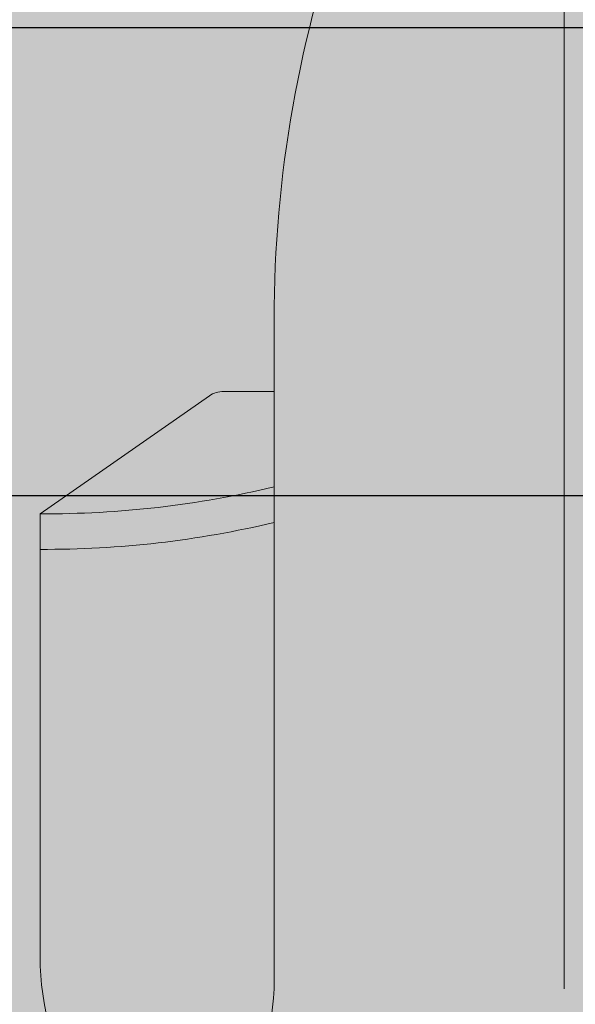
# Model space of a CAD drawing. Units: inches. Extents: x 389 to 971, y 148 to 870.
# Tile 2 of 14: x 500 to 515, y 364 to 389. Entities that reach past the tile are written whole.
import ezdxf

# ---------------------------------------------------------------- set-up
doc = ezdxf.new("R2010")
doc.units = ezdxf.units.IN
doc.header["$MEASUREMENT"] = 0
for name, color, linetype, lineweight in [('A-ANNO-DIMS', 2, 'Continuous', 18), ('C-VEHI', 8, 'Continuous', 13), ('L-GRND-BASE-PATT', 8, 'Continuous', 13)]:
    doc.layers.add(name, color=color, linetype=linetype, lineweight=lineweight)
doc.layers.add('C-VEHI-PATT', color=18, linetype='Continuous', lineweight=13, true_color=0x000000)
doc.layers.add('L-GRND-PATT', color=39, linetype='Continuous', lineweight=13, true_color=0x603913)
doc.styles.get("Standard").update_dxf_attribs({"font": 'arial.ttf'})
doc.dimstyles.get("Standard").update_dxf_attribs({"dimtxt": 8, "dimasz": 8, "dimexe": 0.18, "dimexo": 0.0625, "dimgap": 0.09, "dimtad": 0, "dimtih": 1, "dimtoh": 1, "dimdec": 0, "dimzin": 0, "dimdsep": 46, "dimlunit": 3, "dimtxsty": 'Standard', "dimcen": 0.09, "dimadec": 0, "dimazin": 0, "dimtfac": 1, "dimtdec": 0, "dimtofl": 0, "dimtmove": 0, "dimatfit": 3, "dimfxl": 1, "dimtolj": 1, "dimtzin": 0, "dimarcsym": 0})

# ---------------------------------------------------------------- blocks, each defined once
blk = doc.blocks.new('*U7')
for p, q in [((-4.43e-14, -2.558e-13), (51.68362801571248, -2.558e-13)), ((29.77279020470884, -9.50583338362054), (51.68362801571248, -9.50583338362054)), ((32.12291633764599, -9.50583338362054), (32.12291633764599, -11.15369945057762)), ((32.26591480791686, -11.62530558863292), (36.12873726252356, -17.16961494239257)), ((36.12873726252356, -17.16961494239257), (50.93891189819171, -17.16961494239257))]:
    blk.add_line(p, q)
for centre, major_axis, ratio, start_param, end_param in [((29.77279020470884, -46.66302566589627), (5.12e-14, 56.16885904951626), 0.842303869543976, 7e-16, 0.5903187773915901), ((29.77279020470884, 46.66302566589578), (4.004e-13, 56.16885904951626), 0.8423038695439734, 2.55127387619821, 3.141592653589801), ((13.03653510440275, -17.00972444508983), (1.2568e-12, -27.41599049210552), 0.8423038695439318, 1.564964277657711, 1.848039256919935), ((14.20086229321332, -17.00972444508983), (1.2568e-12, -27.41599049210552), 0.8423038695439318, 1.564964277657711, 1.848039256919935), ((32.74615637525823, -11.1536994505777), (1.3e-13, -0.7399230374541176), 0.8423038695439093, 4.712388980384541, 5.403471737230034)]:
    blk.add_ellipse(centre, major_axis=major_axis, ratio=ratio, start_param=start_param, end_param=end_param)
at = {"extrusion": (0, 0, -1)}
blk.add_ellipse((50.7902773840875, -13.33772416300655), major_axis=(6.340077547122382, 0.3566085810370246), ratio=0.6038335755719145, start_param=-1.39555193967809, end_param=1.581314658479915, dxfattribs=at)
blk = doc.blocks.new('*D53')
at = {"layer": 'A-ANNO-DIMS', "color": 0, "lineweight": -2, "transparency": 16777216}
for p, q in [((397.8910240000004, 396.9189020000002), (397.8910240000004, 404.9189020000001)), ((690.1535240000002, 388.9189020000003), (397.7110240000004, 388.9189020000002)), ((690.1535240000002, 376.9189020000001), (397.7110240000005, 376.9189020000001)), ((397.8910240000005, 368.9189020000001), (397.8910240000005, 360.918902))]:
    blk.add_line(p, q, dxfattribs=at)
at = {"layer": 'A-ANNO-DIMS', "color": 0, "transparency": 16777216}
for points in [[(396.5576906666671, 396.9189020000002), (399.2243573333337, 396.9189020000002), (397.8910240000004, 388.9189020000002)], [(396.5576906666671, 368.9189020000001), (399.2243573333338, 368.9189020000001), (397.8910240000005, 376.9189020000001)]]:
    blk.add_solid(points, dxfattribs=at)
at = {"layer": 'Defpoints', "color": 0, "transparency": 16777216}
for p in [(397.8910240000004, 388.9189020000002), (690.2160240000001, 388.9189020000003), (690.2160240000001, 376.9189020000001)]:
    blk.add_point(p, dxfattribs=at)
at = {"layer": 'A-ANNO-DIMS', "color": 0, "transparency": 16777216, "insert": (397.8910240000004, 382.9189019999999), "char_height": 8, "attachment_point": 5}
blk.add_mtext('\\A1;12', dxfattribs=at)

msp = doc.modelspace()

# ---------------------------------------------------------------- hatches: boundary and pattern name
at = {"layer": 'C-VEHI-PATT'}
h = msp.add_hatch(color=256, dxfattribs=at)
h.dxf.hatch_style = 1
edge = h.paths.add_edge_path()
edge.add_ellipse((550.9021553826709, 381.4331108862803), major_axis=(-43.99405423656321, 1.9369e-12), ratio=0.8423038695439613, start_angle=-29.43856959797762, end_angle=1.8189894035458565e-12, ccw=False)
edge.add_line((514.3535105156315, 402.059641051582), (514.3535105156315, 404.7525403567118))
edge.add_ellipse((514.3535105156316, 404.2643898676136), major_axis=(0.5795420236673633, 2e-16), ratio=0.8423038695437671, start_angle=90.00000000001334, end_angle=127.9331304598466)
edge.add_line((514.0354569934393, 404.6724605914631), (509.5535496243029, 402.1940957519602))
edge.add_ellipse((473.3138688667988, 564.9222417143382), major_axis=(196.5636751472093, 8.4793e-12), ratio=0.8423038695439335, start_angle=-80.7434339928015, end_angle=-77.44506735586577, ccw=False)
edge.add_ellipse((535.9119176052684, 201.7546502845751), major_axis=(239.1273775699096, 1.008988e-10), ratio=0.842303869543627, start_angle=100.2095389971183, end_angle=102.4446272934191)
edge.add_ellipse((979.5722266908713, 375.4013592680145), major_axis=(-488.2195497741742, 7.7268e-12), ratio=0.842303869543895, start_angle=-2.863714607837472, end_angle=2.198540565955285)
edge.add_ellipse((510.1338164488812, 299.4839331720496), major_axis=(70.3178640738586, 3.814e-12), ratio=0.8423038695439212, start_angle=94.08241069114638, end_angle=107.71995322274631, ccw=False)
edge.add_line((505.914122382133, 358.6062023341113), (522.79289864913, 358.606202334111))
edge.add_ellipse((518.5732045823792, 299.4839331720493), major_axis=(-70.31786407385354, 1.4408e-12), ratio=0.8423038695439844, start_angle=252.2800467772501, end_angle=265.91758930884987, ccw=False)
edge.add_ellipse((49.13479434038987, 375.4013592680261), major_axis=(-488.2195497741754, 2.5232e-12), ratio=0.8423038695439587, start_angle=177.8014594340444, end_angle=182.8637146078372)
edge.add_ellipse((492.795103425985, 201.7546502845724), major_axis=(239.12737756976, 4.82267e-11), ratio=0.8423038695441539, start_angle=77.5553727065425, end_angle=79.79046100284327)
edge.add_ellipse((555.3931521644682, 564.9222417143374), major_axis=(-196.5636751472384, 3.62381e-11), ratio=0.8423038695438114, start_angle=77.4450673558726, end_angle=80.74343399280832, ccw=False)
edge.add_line((519.1534714069603, 402.19409575196), (514.671564037824, 404.6724605914631))
edge.add_ellipse((514.3535105156316, 404.2643898676136), major_axis=(0.5795420236673633, 2e-16), ratio=0.8423038695437671, start_angle=52.06686954015338, end_angle=90.00000000001334)
edge.add_line((514.3535105156315, 404.7525403567118), (514.3535105156315, 402.0596410515821))
edge.add_ellipse((477.8048656485917, 381.4331108862812), major_axis=(-43.99405423656326, 6.67e-13), ratio=0.8423038695439753, start_angle=180.0000000000002, end_angle=209.4385695979796, ccw=False)
edge.add_line((521.7989198851549, 381.4331108862806), (521.7989198851549, 379.5923831537828))
edge.add_line((521.7989198851549, 379.5923831537828), (523.2258361412675, 379.5923831537828))
edge.add_ellipse((523.0896049791924, 379.1042326646847), major_axis=(0.5795420236669786, 3.601e-13), ratio=0.8423038695443263, start_angle=45.519789117397124, end_angle=89.99999999996442, ccw=False)
edge.add_line((523.4589887688404, 379.4803801228631), (527.8015488731598, 376.4548385069232))
edge.add_line((527.8015488731598, 376.4548385069232), (527.8015488731597, 364.8548231745798))
edge.add_ellipse((524.8002343791572, 364.9712406163019), major_axis=(0.279312372030448, 4.96584264291768), ratio=0.6038335755719146, start_angle=106.34259195429831, end_angle=270.9979857249735, ccw=False)
edge.add_line((521.7989198851548, 364.2715269884119), (521.7989198851549, 381.4331108862806))
edge.add_ellipse((477.8048656485917, 381.4331108862812), major_axis=(-43.99405423656326, 6.67e-13), ratio=0.8423038695439753, start_angle=180.0000000000001, end_angle=209.4385695979795)
edge.add_ellipse((550.9021553826709, 381.4331108862803), major_axis=(-43.99405423656321, 1.9369e-12), ratio=0.8423038695439613, start_angle=-29.43856959797755, end_angle=1.8539e-12)
edge.add_line((506.9081011461076, 381.43311088628), (506.9081011461074, 364.2715269884121))
edge.add_ellipse((503.9067866521049, 364.9712406163021), major_axis=(-0.2793123720310282, 4.965842642917721), ratio=0.6038335755718928, start_angle=89.00201427501901, end_angle=253.6574080456941, ccw=False)
edge.add_line((500.9054721581025, 364.8548231745812), (500.9054721581025, 376.4548385069235))
edge.add_line((500.9054721581025, 376.4548385069235), (505.3530060491612, 379.5535172937331))
edge.add_ellipse((505.61741605207, 379.1042326646849), major_axis=(-0.5795420236672051, 1.236e-13), ratio=0.842303869543997, start_angle=-89.99999999998778, end_angle=-45.51978911742469, ccw=False)
edge.add_line((505.61741605207, 379.5923831537831), (506.9081011461076, 379.5923831537831))
edge.add_line((506.9081011461076, 379.5923831537831), (506.9081011461076, 381.43311088628))
h = msp.add_hatch(color=256, dxfattribs=at)
h.dxf.hatch_style = 1
edge = h.paths.add_edge_path()
edge.add_ellipse((550.9021553826709, 381.4331108862803), major_axis=(-43.99405423656321, 1.9369e-12), ratio=0.8423038695439613, start_angle=-17.01851281727818, end_angle=1.8189894035458565e-12, ccw=False)
edge.add_line((509.5535496243029, 394.0892586662828), (509.5535496243029, 402.1940957519602))
edge.add_ellipse((473.3138688667988, 564.9222417143382), major_axis=(196.5636751472093, 8.4793e-12), ratio=0.8423038695439335, start_angle=-80.7434339928015, end_angle=-77.44506735586577, ccw=False)
edge.add_ellipse((535.9119176052684, 201.7546502845751), major_axis=(239.1273775699096, 1.008988e-10), ratio=0.842303869543627, start_angle=100.2095389971183, end_angle=102.4446272934191)
edge.add_ellipse((979.5722266908713, 375.4013592680145), major_axis=(-488.2195497741742, 7.7268e-12), ratio=0.842303869543895, start_angle=-2.863714607837472, end_angle=2.198540565955285)
edge.add_ellipse((510.1338164488812, 299.4839331720496), major_axis=(70.3178640738586, 3.814e-12), ratio=0.8423038695439212, start_angle=94.08241069114638, end_angle=107.71995322274631, ccw=False)
edge.add_line((505.914122382133, 358.6062023341113), (509.5535496243029, 358.6062023341112))
edge.add_line((509.5535496243029, 358.6062023341112), (509.5535496243029, 394.0892586662828))
edge.add_ellipse((550.9021553826709, 381.4331108862803), major_axis=(-43.99405423656321, 1.9369e-12), ratio=0.8423038695439613, start_angle=-17.01851281727824, end_angle=1.8539e-12)
edge.add_line((506.9081011461076, 381.43311088628), (506.9081011461074, 364.2715269884121))
edge.add_ellipse((503.9067866521049, 364.9712406163021), major_axis=(-0.2793123720310282, 4.965842642917721), ratio=0.6038335755718928, start_angle=89.00201427501901, end_angle=253.6574080456941, ccw=False)
edge.add_line((500.9054721581025, 364.8548231745812), (500.9054721581025, 376.4548385069235))
edge.add_line((500.9054721581025, 376.4548385069235), (505.3172273641584, 379.5285896248376))
edge.add_ellipse((505.61741605207, 379.1042326646849), major_axis=(-0.5795420236672051, 1.236e-13), ratio=0.842303869543997, start_angle=-89.99999999998778, end_angle=-45.51978911742469, ccw=False)
edge.add_line((505.61741605207, 379.5923831537831), (506.9081011461076, 379.5923831537831))
edge.add_line((506.9081011461076, 379.5923831537831), (506.9081011461076, 381.43311088628))
h = msp.add_hatch(color=256, dxfattribs=at)
h.dxf.hatch_style = 1
edge = h.paths.add_edge_path(flags=16)
edge.add_ellipse((3386.011413077446, 329.726312794031), major_axis=(-2896.629999631248, 1.069454e-10), ratio=0.8423038695494893, start_angle=-0.1208973690315247, end_angle=0.3640763488915013, ccw=False)
edge.add_line((489.3905023836935, 335.8383575186984), (486.2179253655185, 346.1978202249628))
edge.add_ellipse((8782.002602781096, 354.247254279773), major_axis=(-8295.790181758603, 9.87839e-10), ratio=0.8423038695486498, start_angle=0.0555943135052214, end_angle=0.3777641939157137)
edge.add_line((486.4665645878948, 299.5520931219791), (489.4638383140943, 311.3204429697198))
edge = h.paths.add_edge_path(flags=16)
edge.add_ellipse((512.1608573463288, 287.5825181681774), major_axis=(62.33048198263887, 2.0798e-12), ratio=0.8423038695439498, start_angle=94.8700695971331, end_angle=112.791914877584)
edge.add_line((491.3642517254777, 337.0752369161335), (489.6529508739416, 349.9015767089268))
edge.add_ellipse((510.1338164488795, 298.7862183048575), major_axis=(64.04807894948699, 3.9006e-12), ratio=0.8423038695439252, start_angle=94.27742096304979, end_angle=111.83495379670401, ccw=False)
edge.add_line((506.1068129054811, 352.6274231954524), (522.600208125781, 352.6274231954521))
edge.add_ellipse((518.5732045823798, 298.7862183048586), major_axis=(64.04807894948067, 3.24e-14), ratio=0.8423038695439885, start_angle=68.16504620328948, end_angle=85.72257903694378, ccw=False)
edge.add_line((539.05407015732, 349.9015767089259), (537.3427693057835, 337.0752369161327))
edge.add_ellipse((516.5461636849332, 287.5825181681899), major_axis=(62.33048198262021, 1.5954e-12), ratio=0.8423038695439995, start_angle=67.20808512240782, end_angle=85.12993040286212)
edge.add_line((521.0080028322477, 339.9490379899644), (507.6990181990146, 339.9490379899646))
edge = h.paths.add_edge_path(flags=16)
edge.add_ellipse((514.3535105156315, 391.3730654902235), major_axis=(-115.1512533244504, 1.8736e-12), ratio=0.8423038695439684, start_angle=76.4018653097696, end_angle=103.5981346902308)
edge.add_line((537.3427693057832, 296.3333211885938), (537.342769305783, 281.5897392316151))
edge.add_ellipse((514.3535105156313, 376.6294835332447), major_axis=(-115.1512533244486, 9.02e-13), ratio=0.8423038695439828, start_angle=76.40186530976922, end_angle=103.59813469023032, ccw=False)
edge.add_line((491.3642517254773, 281.5897392316156), (491.3642517254774, 296.3333211885945))
edge = h.paths.add_edge_path()
edge.add_ellipse((8782.002602781105, 354.2472542798386), major_axis=(-8296.949265805946, 5.39345e-11), ratio=0.8423038695428886, start_angle=0.3838667787920247, end_angle=0.5282714718170651)
edge.add_ellipse((8782.002602781105, 354.2472542798386), major_axis=(-8296.949265805946, 5.39345e-11), ratio=0.8423038695428886, start_angle=0.5282714718170651, end_angle=0.6465540970606384)
edge.add_ellipse((488.1158467995968, 260.6509346628684), major_axis=(2.318168094668909, 7.48e-14), ratio=0.8423038695439647, start_angle=180.6465540970884, end_angle=269.9999999999081)
edge.add_line((488.115846799593, 258.6983327064755), (491.3642517254771, 258.6983327064753))
edge.add_line((491.3642517254771, 258.6983327064753), (491.3642517254771, 274.201106836649))
edge.add_ellipse((493.6824198201462, 273.9438556676354), major_axis=(-2.318168094668919, 1.896e-13), ratio=0.8423038695439611, start_angle=-89.99999999999523, end_angle=4.718003765447065e-12, ccw=False)
edge.add_line((493.6824198201462, 275.8964576240284), (535.3300149439905, 275.8964576240277))
edge.add_ellipse((535.024601211114, 273.9438556676347), major_axis=(2.318168094668976, 2.946e-13), ratio=0.8423038695439647, start_angle=-7.275957614183426e-12, end_angle=89.99999999998943, ccw=False)
edge.add_line((537.342769305783, 273.9438556676347), (537.3427693057827, 258.698332706474))
edge.add_line((537.3427693057827, 258.698332706474), (540.591174231666, 258.6983327064739))
edge.add_ellipse((540.5911742316634, 260.6509346628669), major_axis=(-2.318168094668839, 2.143e-13), ratio=0.8423038695440144, start_angle=90.00000000008203, end_angle=179.3534459029346)
edge.add_ellipse((-7753.295581726658, 354.2472542799028), major_axis=(-8296.949265782761, 2.068448e-10), ratio=0.8423038695442414, start_angle=179.3534459029388, end_angle=179.3813568036815)
edge.add_ellipse((-7753.295581726658, 354.2472542799028), major_axis=(-8296.949265782761, 2.068448e-10), ratio=0.8423038695442414, start_angle=179.3813568036815, end_angle=179.4717285281828)
edge.add_ellipse((-7753.295581726658, 354.2472542799028), major_axis=(-8296.949265782761, 2.068448e-10), ratio=0.8423038695442414, start_angle=179.4717285281828, end_angle=179.6161332212082)
edge.add_ellipse((-7753.295581726658, 354.2472542799028), major_axis=(-8296.949265782761, 2.068448e-10), ratio=0.8423038695442414, start_angle=179.6161332212082, end_angle=180.090229088595)
edge.add_ellipse((-7753.295581726658, 354.2472542799028), major_axis=(-8296.949265782761, 2.068448e-10), ratio=0.8423038695442414, start_angle=180.090229088595, end_angle=180.134986576859)
edge.add_ellipse((129.8867725257751, 372.4897205359271), major_axis=(-413.7373561031673, 2.44623e-11), ratio=0.8423038695441432, start_angle=180.1806905311865, end_angle=182.1799503136479)
edge.add_ellipse((129.8867725257751, 372.4897205359271), major_axis=(-413.7373561031673, 2.44623e-11), ratio=0.8423038695441432, start_angle=182.1799503136479, end_angle=183.6504275857017)
edge.add_ellipse((492.7951034259847, 196.3854951855023), major_axis=(245.3971626940514, 1.422861e-10), ratio=0.8423038695444116, start_angle=76.21947101046817, end_angle=77.87403444768196)
edge.add_ellipse((49.13479434038987, 375.4013592680261), major_axis=(-488.2195497741754, 2.5232e-12), ratio=0.8423038695439587, start_angle=177.8014594340445, end_angle=182.8637146078372, ccw=False)
edge.add_ellipse((518.5732045823792, 299.4839331720493), major_axis=(-70.31786407385354, 1.4408e-12), ratio=0.8423038695439844, start_angle=252.2800467772501, end_angle=265.9175893088498)
edge.add_line((522.79289864913, 358.606202334111), (505.9141223821329, 358.6062023341113))
edge.add_ellipse((510.1338164488812, 299.4839331720496), major_axis=(70.3178640738586, 3.814e-12), ratio=0.8423038695439212, start_angle=94.08241069114636, end_angle=107.7199532227462)
edge.add_ellipse((979.5722266908713, 375.4013592680145), major_axis=(-488.2195497741742, 7.7268e-12), ratio=0.842303869543895, start_angle=-2.863714607837494, end_angle=2.198540565955284, ccw=False)
edge.add_ellipse((535.9119176052733, 196.3854951855018), major_axis=(-245.3971626940985, 1.013648e-10), ratio=0.8423038695442548, start_angle=-77.87403444769295, end_angle=-76.2194710104792)
edge.add_ellipse((898.8202485054873, 372.489720535918), major_axis=(413.7373561031672, 1.26113e-11), ratio=0.8423038695441164, start_angle=176.3495724142985, end_angle=177.8200496863523)
edge.add_ellipse((898.8202485054873, 372.489720535918), major_axis=(413.7373561031672, 1.26113e-11), ratio=0.8423038695441164, start_angle=177.8200496863523, end_angle=179.8643876095591)
edge.add_ellipse((8782.002602781105, 354.2472542798386), major_axis=(-8296.949265805946, 5.39345e-11), ratio=0.8423038695428886, start_angle=-0.1349865768573029, end_angle=-0.090229088593484)
edge.add_ellipse((8782.002602781105, 354.2472542798386), major_axis=(-8296.949265805946, 5.39345e-11), ratio=0.8423038695428886, start_angle=-0.090229088593484, end_angle=0.3838667787920247)
edge = h.paths.add_edge_path(flags=16)
edge.add_ellipse((-2357.304392046186, 329.7263127941099), major_axis=(2896.629999631251, 5.35614e-11), ratio=0.8423038695445265, start_angle=-0.3640763488920631, end_angle=0.1208973690309369)
edge.add_line((539.3165186475693, 335.8383575187012), (542.4890956657468, 346.1978202249727))
edge.add_ellipse((-7753.295581749842, 354.2472542800017), major_axis=(8295.790181758617, 3.2664368e-09), ratio=0.8423038695525207, start_angle=-0.37776419393310334, end_angle=-0.055594313522590255, ccw=False)
edge.add_line((542.240456443367, 299.5520931219743), (539.2431827171666, 311.3204429697195))
h = msp.add_hatch(color=256, dxfattribs=at)
h.dxf.hatch_style = 1
edge = h.paths.add_edge_path()
edge.add_line((506.9081011461076, 379.5923831537831), (505.61741605207, 379.5923831537831))
edge.add_ellipse((505.61741605207, 379.1042326646849), major_axis=(-0.5795420236672051, 1.236e-13), ratio=0.842303869543997, start_angle=-89.99999999998776, end_angle=-45.51978911742479)
edge.add_line((505.2480322624221, 379.4803801228633), (500.9054721581027, 376.4548385069235))
edge.add_ellipse((501.0307058076602, 394.5417217261546), major_axis=(21.47347468097092, 9.597e-13), ratio=0.8423038695439192, start_angle=269.6032901400189, end_angle=288.6674954926004)
edge.add_line((506.9081011461076, 377.1452135063883), (506.9081011461076, 379.5923831537831))
h = msp.add_hatch(color=256, dxfattribs=at)
h.dxf.hatch_style = 1
edge = h.paths.add_edge_path()
edge.add_line((506.9081011461076, 379.5923831537831), (505.61741605207, 379.5923831537831))
edge.add_ellipse((505.61741605207, 379.1042326646849), major_axis=(-0.5795420236672051, 1.236e-13), ratio=0.842303869543997, start_angle=-89.99999999998776, end_angle=-45.51978911742479)
edge.add_line((505.2480322624221, 379.4803801228633), (500.9054721581027, 376.4548385069235))
edge.add_ellipse((501.0307058076602, 394.5417217261546), major_axis=(21.47347468097092, 9.597e-13), ratio=0.8423038695439192, start_angle=269.6032901400189, end_angle=288.6674954926004)
edge.add_line((506.9081011461076, 377.1452135063883), (506.9081011461076, 379.5923831537831))
h = msp.add_hatch(color=256, dxfattribs=at)
h.dxf.hatch_style = 1
edge = h.paths.add_edge_path()
edge.add_line((506.9081011461076, 379.5923831537831), (505.61741605207, 379.5923831537831))
edge.add_ellipse((505.61741605207, 379.1042326646849), major_axis=(-0.5795420236672051, 1.236e-13), ratio=0.842303869543997, start_angle=-89.99999999998776, end_angle=-45.51978911742479)
edge.add_line((505.2480322624221, 379.4803801228633), (500.9054721581027, 376.4548385069235))
edge.add_ellipse((501.0307058076602, 394.5417217261546), major_axis=(21.47347468097092, 9.597e-13), ratio=0.8423038695439192, start_angle=269.6032901400189, end_angle=288.6674954926004)
edge.add_line((506.9081011461076, 377.1452135063883), (506.9081011461076, 379.5923831537831))
h = msp.add_hatch(color=256, dxfattribs=at)
h.dxf.hatch_style = 1
edge = h.paths.add_edge_path()
edge.add_ellipse((501.0307058076602, 394.5417217261546), major_axis=(21.47347468097092, 9.597e-13), ratio=0.8423038695439192, start_angle=269.60329014001894, end_angle=288.66749549260044, ccw=False)
edge.add_line((500.9054721581025, 376.4548385069235), (500.9054721581025, 375.5428834777413))
edge.add_ellipse((501.0307058076602, 393.6297666969722), major_axis=(-21.47347468096764, 1.6558e-12), ratio=0.8423038695440453, start_angle=89.60329014002593, end_angle=108.6674954926075)
edge.add_line((506.9081011461076, 376.2332584772061), (506.9081011461076, 377.1452135063883))
h = msp.add_hatch(color=256, dxfattribs=at)
h.dxf.hatch_style = 1
edge = h.paths.add_edge_path()
edge.add_ellipse((501.0307058076602, 393.6297666969722), major_axis=(-21.47347468096764, 1.6558e-12), ratio=0.8423038695440453, start_angle=89.60329014002599, end_angle=108.66749549260749, ccw=False)
edge.add_line((500.9054721581025, 375.5428834777413), (500.9054721581025, 364.8548231745812))
edge.add_ellipse((503.9067866521049, 364.9712406163021), major_axis=(-0.2793123720310282, 4.965842642917721), ratio=0.6038335755718928, start_angle=89.0020142750189, end_angle=253.657408045694)
edge.add_line((506.9081011461074, 364.2715269884121), (506.9081011461076, 376.2332584772061))
h = msp.add_hatch(color=256, dxfattribs=at)
h.dxf.hatch_style = 1
edge = h.paths.add_edge_path()
edge.add_ellipse((501.0307058076602, 393.6297666969722), major_axis=(-21.47347468096764, 1.6558e-12), ratio=0.8423038695440453, start_angle=89.60329014002599, end_angle=108.66749549260749, ccw=False)
edge.add_line((500.9054721581025, 375.5428834777413), (500.9054721581025, 364.8548231745812))
edge.add_ellipse((503.9067866521049, 364.9712406163021), major_axis=(-0.2793123720310282, 4.965842642917721), ratio=0.6038335755718928, start_angle=89.0020142750189, end_angle=253.657408045694)
edge.add_line((506.9081011461074, 364.2715269884121), (506.9081011461076, 376.2332584772061))
at = {"layer": 'L-GRND-BASE-PATT'}
h = msp.add_hatch(color=256, dxfattribs=at)
h.dxf.hatch_style = 1
edge = h.paths.add_edge_path(flags=16)
edge.add_ellipse((8782.002602781105, 354.2472542798386), major_axis=(-8296.949265805946, 5.39345e-11), ratio=0.8423038695428886, start_angle=-0.0902290885933894, end_angle=0.3838667787920258, ccw=False)
edge.add_ellipse((485.0533369751568, 368.2895347624687), major_axis=(-1.159084047334488, 1.838e-13), ratio=0.8423038695439892, start_angle=9.094947017729282e-12, end_angle=90.00000000000898, ccw=False)
edge.add_line((483.8942529278224, 368.2895347624687), (483.8942529278225, 387.6039063360424))
edge.add_ellipse((485.0533369751571, 387.2465553762829), major_axis=(1.159084047334488, 1.838e-13), ratio=0.8423038695439892, start_angle=89.99999999999102, end_angle=179.9999999999909, ccw=False)
edge.add_line((485.0533369751572, 388.2228563544795), (485.5047440247956, 388.2228563544795))
edge.add_ellipse((898.8202485054873, 372.489720535918), major_axis=(413.7373561031672, 1.26113e-11), ratio=0.8423038695441164, start_angle=176.3495724142986, end_angle=177.8200496863524, ccw=False)
edge.add_ellipse((535.9119176052733, 196.3854951855018), major_axis=(-245.3971626940985, 1.013648e-10), ratio=0.8423038695442548, start_angle=-77.87403444769302, end_angle=-76.2194710104792, ccw=False)
edge.add_ellipse((535.9119176052684, 201.7546502845751), major_axis=(239.1273775699096, 1.008988e-10), ratio=0.842303869543627, start_angle=100.20953899711827, end_angle=102.44462729341922, ccw=False)
edge.add_ellipse((473.3138688667988, 564.9222417143382), major_axis=(196.5636751472093, 8.4793e-12), ratio=0.8423038695439335, start_angle=-80.74343399280163, end_angle=-77.44506735586587)
edge.add_line((509.5535496243029, 402.1940957519602), (514.3535105156315, 404.8483349684994))
edge.add_line((514.3535105156315, 404.8483349684994), (514.3535105156315, 404.7971763262221))
edge.add_ellipse((514.3535105156316, 404.2643898676136), major_axis=(0.5795420236673633, 2e-16), ratio=0.8423038695437671, start_angle=52.06686954015339, end_angle=90.00000000001342, ccw=False)
edge.add_line((514.671564037824, 404.672460591463), (519.1534714069603, 402.19409575196))
edge.add_ellipse((555.3931521644682, 564.9222417143374), major_axis=(-196.5636751472384, 3.62381e-11), ratio=0.8423038695438114, start_angle=77.44506735587258, end_angle=80.74343399280833)
edge.add_ellipse((492.795103425985, 201.7546502845724), major_axis=(239.12737756976, 4.82267e-11), ratio=0.8423038695441539, start_angle=77.55537270654253, end_angle=79.7904610028433, ccw=False)
edge.add_ellipse((492.7951034259847, 196.3854951855023), major_axis=(245.3971626940514, 1.422861e-10), ratio=0.8423038695444116, start_angle=76.21947101046823, end_angle=77.87403444768199, ccw=False)
edge.add_ellipse((129.8867725257751, 372.4897205359271), major_axis=(-413.7373561031673, 2.44623e-11), ratio=0.8423038695441432, start_angle=182.179950313648, end_angle=183.6504275857018, ccw=False)
edge.add_line((543.2022770064673, 388.2228563544788), (544.0779382625514, 388.2228563544787))
edge.add_ellipse((543.6536840561057, 387.2465553762822), major_axis=(-1.159084047334545, 1.527e-13), ratio=0.8423038695438989, start_angle=180.0000000000075, end_angle=270.00000000000756, ccw=False)
edge.add_line((544.8127681034401, 387.2465553762826), (544.8127681034399, 367.9321838027083))
edge.add_ellipse((543.6536840561054, 368.2895347624679), major_axis=(1.159084047334544, 7.24e-14), ratio=0.8423038695439478, start_angle=269.9999999999964, end_angle=359.9999999999964, ccw=False)
edge.add_ellipse((-7753.295581726658, 354.2472542799028), major_axis=(-8296.949265782761, 2.068448e-10), ratio=0.8423038695442414, start_angle=179.6161332212083, end_angle=180.0902290885951, ccw=False)
edge.add_line((543.3912265319653, 298.6607849184036), (544.0779382625504, 298.6607849184036))
edge.add_ellipse((543.6536840561046, 297.6844839402071), major_axis=(1.159084047334431, 1.769e-13), ratio=0.8423038695439814, start_angle=-1.1482370609883219e-11, end_angle=89.99999999999119, ccw=False)
edge.add_line((544.8127681034391, 297.684483940207), (544.8127681034387, 278.3701123666333))
edge.add_ellipse((543.6536840561043, 278.727463326393), major_axis=(-1.159084047334431, 2.574e-13), ratio=0.8423038695440306, start_angle=90.00000000001268, end_angle=180.0000000000099, ccw=False)
edge.add_line((543.6536840561045, 277.7511623481965), (543.1566278692261, 277.7511623481965))
edge.add_ellipse((-7753.295581726658, 354.2472542799028), major_axis=(-8296.949265782761, 2.068448e-10), ratio=0.8423038695442414, start_angle=179.3813568036816, end_angle=179.4717285281829, ccw=False)
edge.add_ellipse((542.4236240941387, 263.2762864208561), major_axis=(-1.738626071001761, 2.132e-13), ratio=0.8423038695439151, start_angle=179.3717627838137, end_angle=248.464756601011, ccw=False)
edge.add_ellipse((-7753.875123750511, 354.2472542780016), major_axis=(-8298.740341433751, 2.4782644722e-06), ratio=0.8423038662721074, start_angle=179.3534459200609, end_angle=179.3717628008941, ccw=False)
edge.add_ellipse((540.0116322079951, 260.6509346628677), major_axis=(-4.109243751168186, 2.384e-13), ratio=0.842303869543976, start_angle=90.0000000000635, end_angle=179.3534459029233, ccw=False)
edge.add_line((540.0116322079991, 257.1897027503593), (488.6953888232593, 257.1897027503609))
edge.add_ellipse((488.6953888232669, 260.6509346628715), major_axis=(4.10924375117072, 1.262e-13), ratio=0.8423038695439824, start_angle=180.6465540970565, end_angle=269.9999999998589, ccw=False)
edge.add_ellipse((8782.582144816053, 354.2472542821698), major_axis=(-8298.740341477976, 1.8591886369e-06), ratio=0.8423038720186145, start_angle=0.6282372290784792, end_angle=0.6465541099116194, ccw=False)
edge.add_ellipse((486.2833969371199, 263.2762864208594), major_axis=(-1.738626071002378, 2.7e-13), ratio=0.8423038695439394, start_angle=-68.46475649596817, end_angle=0.6282372161796275, ccw=False)
edge.add_ellipse((8782.002602781105, 354.2472542798386), major_axis=(-8296.949265805946, 5.39345e-11), ratio=0.8423038695428886, start_angle=0.5282714718171064, end_angle=0.6465540970606867, ccw=False)
edge.add_line((485.5503931620382, 277.7511623481972), (484.6290827687102, 277.7511623481972))
edge.add_ellipse((485.0533369751559, 278.7274633263938), major_axis=(-1.159084047334545, 3.11e-13), ratio=0.8423038695439968, start_angle=1.5404566511278972e-11, end_angle=90.000000000012, ccw=False)
edge.add_line((483.8942529278214, 278.7274633263938), (483.8942529278216, 298.0418348999672))
edge.add_ellipse((485.053336975156, 297.6844839402078), major_axis=(1.159084047334488, 1.025e-13), ratio=0.8423038695440382, start_angle=89.99999999999488, end_angle=179.9999999999949, ccw=False)
edge = h.paths.add_edge_path(flags=0)
edge.add_ellipse((8782.002602781096, 354.247254279773), major_axis=(-8295.790181758603, 9.87839e-10), ratio=0.8423038695486498, start_angle=0.05559431350519617, end_angle=0.37776419391582294, ccw=False)
edge.add_line((486.2179253655185, 346.1978202249628), (489.3905023836935, 335.8383575186984))
edge.add_ellipse((3386.011413077446, 329.726312794031), major_axis=(-2896.629999631248, 1.069454e-10), ratio=0.8423038695494893, start_angle=-0.1208973690315206, end_angle=0.3640763488915184)
edge.add_line((489.4638383140943, 311.3204429697198), (486.4665645878948, 299.5520931219791))
edge = h.paths.add_edge_path(flags=0)
edge.add_ellipse((514.3535105156315, 391.3730654902235), major_axis=(-115.1512533244504, 1.8736e-12), ratio=0.8423038695439684, start_angle=76.4018653097696, end_angle=103.5981346902308)
edge.add_line((537.3427693057832, 296.3333211885938), (537.342769305783, 281.5897392316151))
edge.add_ellipse((514.3535105156313, 376.6294835332447), major_axis=(-115.1512533244486, 9.02e-13), ratio=0.8423038695439828, start_angle=76.40186530976922, end_angle=103.59813469023032, ccw=False)
edge.add_line((491.3642517254773, 281.5897392316156), (491.3642517254774, 296.3333211885945))
edge = h.paths.add_edge_path(flags=0)
edge.add_line((491.3642517254777, 337.0752369161334), (489.6529508739416, 349.9015767089268))
edge.add_ellipse((510.1338164488795, 298.7862183048575), major_axis=(64.04807894948699, 3.9006e-12), ratio=0.8423038695439252, start_angle=94.27742096304979, end_angle=111.83495379670401, ccw=False)
edge.add_line((506.106812905481, 352.6274231954524), (522.600208125781, 352.6274231954521))
edge.add_ellipse((518.5732045823798, 298.7862183048586), major_axis=(64.04807894948067, 3.24e-14), ratio=0.8423038695439885, start_angle=68.16504620328948, end_angle=85.72257903694378, ccw=False)
edge.add_line((539.05407015732, 349.9015767089259), (537.3427693057835, 337.0752369161327))
edge.add_ellipse((516.5461636849332, 287.5825181681899), major_axis=(62.33048198262021, 1.5954e-12), ratio=0.8423038695439995, start_angle=67.20808512240782, end_angle=85.12993040286212)
edge.add_line((521.0080028322477, 339.9490379899644), (507.6990181990146, 339.9490379899646))
edge.add_ellipse((512.1608573463288, 287.5825181681774), major_axis=(62.33048198263887, 2.0798e-12), ratio=0.8423038695439498, start_angle=94.8700695971331, end_angle=112.791914877584)
edge = h.paths.add_edge_path(flags=0)
edge.add_ellipse((493.6824198201462, 273.9438556676354), major_axis=(-2.318168094668919, 1.896e-13), ratio=0.8423038695439611, start_angle=-89.99999999999523, end_angle=4.718003765447065e-12, ccw=False)
edge.add_line((493.6824198201462, 275.8964576240284), (535.3743409680425, 275.8964576240277))
edge.add_ellipse((535.024601211114, 273.9438556676347), major_axis=(2.318168094668976, 2.946e-13), ratio=0.8423038695439647, start_angle=-7.275957614183426e-12, end_angle=89.99999999998943, ccw=False)
edge.add_line((537.342769305783, 273.9438556676347), (537.3427693057827, 258.698332706474))
edge.add_line((537.3427693057827, 258.698332706474), (540.5911742316662, 258.6983327064739))
edge.add_ellipse((540.5911742316634, 260.6509346628669), major_axis=(-2.318168094668839, 2.143e-13), ratio=0.8423038695440144, start_angle=90.00000000008203, end_angle=179.3534459029346)
edge.add_line((540.5911742316662, 258.6983327064739), (487.7691399811528, 258.6983327064755))
edge.add_ellipse((488.1158467995968, 260.6509346628684), major_axis=(2.318168094668909, 7.48e-14), ratio=0.8423038695439647, start_angle=180.6465540970884, end_angle=269.9999999999081)
edge.add_line((488.1158467995931, 258.6983327064755), (491.3642517254771, 258.6983327064754))
edge.add_line((491.3642517254771, 258.6983327064754), (491.3642517254771, 274.2384428182294))
h.paths.add_polyline_path([(746.1375687288224, 327.3223047166553), (750.1400147212453, 327.3223047166553), (750.1400147212453, 326.2830696147227), (798.1693712998389, 326.2830696147227), (798.1693712998389, 327.3223047166553), (802.1718172922616, 327.3223047166553), (802.1718172922616, 309.9783792024682, -0.1904762075443491), (746.1375687288224, 309.9783668090107)], flags=16)
h.paths.add_polyline_path([(782.1595875801748, 313.5684994305933), (782.1595893317732, 309.0414930416419, -0.0496282101666581), (766.1497986905329, 309.0414910503953), (766.1498004421323, 313.5684994305933)], flags=0)
h.paths.add_polyline_path([(755.1858908233534, 344.9352232902417), (755.1858908233534, 373.916311072083), (788.1243995226009, 373.916311072083), (788.1243995226009, 344.9352232902417)], flags=16)
h.paths.add_polyline_path([(757.1858908233535, 346.9352232902417), (757.1858908233535, 371.916311072083), (786.1243995226009, 371.916311072083), (786.1243995226009, 346.9352232902417)], flags=0)
h.paths.add_polyline_path([(803.6445810111745, 338.4878931208803), (803.6445810111745, 342.4903391133031), (804.6838161131072, 342.4903391133031), (804.6838161131072, 390.5196956918968), (803.6445810111748, 390.5196956918968), (803.6445810111748, 394.5221416843196), (820.9885065253617, 394.5221416843196, -0.1904762075443491), (820.9885189188192, 338.4878931208803)], flags=16)
h.paths.add_polyline_path([(806.8706930931005, 326.6963103558256), (806.4254411777042, 327.1415622712219), (806.4723791864895, 326.6297175483474)], flags=16)
h.paths.add_polyline_path([(822.0328146004263, 317.4007976138144), (822.1941503181826, 317.8932883068639), (821.562628166435, 317.9885306563034)], flags=16)
h.paths.add_polyline_path([(817.3983862972365, 358.5001248341902), (817.3983862972365, 374.5099119722327), (821.9253926861879, 374.5099137238312, -0.049628210166658), (821.9253946774346, 358.5001230825909)], flags=0)
h.paths.add_polyline_path([(808.1446344648577, 418.9736619306146), (808.2246858861593, 418.5632188717996), (808.5395491501399, 418.5787472453325)], flags=16)
h.paths.add_polyline_path([(820.3158762739024, 412.6690288868844), (820.4772119916585, 413.161519579934), (819.8456898399113, 413.2567619293735)], flags=16)
h.paths.add_polyline_path([(466.3155093563569, 235.5246322146605), (517.3806533266912, 235.5246322146605), (517.3806533266912, 244.4269231682286), (466.3155093563569, 244.4269231682286)], flags=24)
h.paths.add_polyline_path([(739.8737195480014, 256.2000079819968), (815.4040239338423, 256.2000079819968), (815.4040239338423, 265.3453807094367), (739.8737195480014, 265.3453807094367)], flags=24)
h.paths.add_polyline_path([(750.6081538187397, 393.6666679930368), (791.5680640722773, 393.6666679930368), (791.5680640722773, 412.3933175868746), (750.6081538187397, 412.3933175868746)], flags=24)
h.paths.add_polyline_path([(438.9630812812552, 410.0618566955462), (484.6203810968238, 410.0618566955462), (484.6203810968238, 429.1217352891893), (438.9630812812552, 429.1217352891893)], flags=24)
edge = h.paths.add_edge_path()
edge.add_line((839.2160244416713, 285.6445131961097), (611.8786784019748, 285.6445131961099))
edge.add_line((611.8786784019748, 285.6445131961099), (604.3870116090119, 285.6445131961097))
edge.add_line((604.3870116090119, 285.6445131961097), (595.3870116090119, 285.6445131961097))
edge.add_line((595.3870116090119, 285.6445131961097), (595.3870116090118, 370.1553848722774))
edge.add_line((595.3870116090118, 370.1553848722774), (604.0816928471932, 370.1553848722774))
edge.add_line((604.0816928471932, 370.1553848722774), (604.0816928471932, 371.3788335667469))
edge.add_line((604.0816928471932, 371.3788335667469), (632.0194586761203, 371.3788335667469))
edge.add_arc((604.0816928471932, 370.1553848722773), 27.96454158787471, 2.507490703587644, 90.00000000000003)
edge.add_line((604.0816928471932, 398.1199264601519), (599.8870116090108, 398.1652144688576))
edge.add_line((599.8870116090108, 398.1652144688576), (604.4225424425357, 398.1652144688576))
edge.add_arc((604.4225424425357, 428.4020866923496), 30.23687222349201, 270.0000000000002, 357.492509296413)
edge.add_line((634.6304631740308, 427.0792235325719), (604.4225424425357, 427.0792235325719))
edge.add_line((604.4225424425357, 427.0792235325719), (604.4225424425357, 428.4020866923497))
edge.add_line((604.4225424425357, 428.4020866923497), (599.8870116090119, 428.4020866923497))
edge.add_line((599.8870116090119, 428.4020866923497), (595.3870116090116, 428.4020866923497))
edge.add_line((595.3870116090116, 428.4020866923497), (595.3870116090118, 434.6445131961097))
edge.add_line((595.3870116090118, 434.6445131961097), (585.0790669792458, 434.6445131961097))
edge.add_line((585.0790669792458, 434.6445131961097), (540.3921730610418, 434.6445131961097))
edge.add_line((540.3921730610418, 434.6445131961097), (526.712508448134, 434.6445131961097))
edge.add_line((526.712508448134, 434.6445131961097), (488.4094553949635, 434.6445131961097))
edge.add_line((488.4094553949635, 434.6445131961097), (432.2160244416713, 434.6445131961097))
edge.add_line((432.2160244416713, 434.6445131961097), (432.2160244416713, 243.6445131961098))
edge.add_line((432.2160244416713, 243.6445131961098), (437.2160244416714, 243.6445131961098))
edge.add_line((437.2160244416714, 243.6445131961098), (437.2160244416714, 234.6445131961098))
edge.add_line((437.2160244416714, 234.6445131961098), (581.2160244416713, 234.6445131961098))
edge.add_line((581.2160244416713, 234.6445131961098), (581.2160244416713, 238.6445131961097))
edge.add_line((581.2160244416713, 238.6445131961097), (581.2160244416713, 243.6445131961098))
edge.add_line((581.2160244416713, 243.6445131961098), (590.2160244416713, 243.6445131961098))
edge.add_line((590.2160244416713, 243.6445131961098), (590.2160244416713, 238.6445131961097))
edge.add_line((590.2160244416713, 238.6445131961097), (839.2160244416713, 238.6445131961098))
edge.add_line((839.2160244416713, 238.6445131961098), (839.2160244416713, 285.6445131961097))
at = {"layer": 'L-GRND-PATT'}
h = msp.add_hatch(dxfattribs=at)
h.set_pattern_fill('EARTH', color=256, angle=45)
h.set_pattern_definition([(45, (0, 0), (0, 8.980256121069154), [6.349999999999999, -6.349999999999999]), (45, (-1.683798022700466, 1.683798022700466), (0, 8.980256121069154), [6.349999999999999, -6.349999999999999]), (45, (-3.367596045400933, 3.367596045400933), (0, 8.980256121069154), [6.349999999999999, -6.349999999999999]), (135, (-3.367596045400933, 4.490128060534576), (-8.980256121069154, 0), [6.349999999999999, -6.349999999999999]), (135, (-1.683798022700466, 6.173926083235043), (-8.980256121069154, 0), [6.349999999999999, -6.349999999999999]), (135, (0, 7.85772410593551), (-8.980256121069154, 0), [6.349999999999999, -6.349999999999999])])
h.paths.add_polyline_path([(432.2160244416713, 243.6445131961098), (437.2160244416714, 243.6445131961098), (437.2160244416714, 234.6445131961098), (581.2160244416713, 234.6445131961098), (581.2160244416713, 238.6445131961097), (581.2160244416713, 243.6445131961098), (590.2160244416713, 243.6445131961098), (590.2160244416713, 238.6445131961097), (839.2160244416713, 238.6445131961098), (839.2160244416712, 285.6445131961097), (810.0513609197296, 285.6445131961097), (733.8056934525983, 285.6445131961099), (684.2433676403508, 285.6445131961098), (611.8786784019748, 285.6445131961099), (604.3870116090119, 285.6445131961097), (595.3870116090119, 285.6445131961097), (595.3870116090118, 370.1553848722774), (604.0816928471932, 370.1553848722774), (604.0816928471932, 371.3788335667469), (632.0194586761203, 371.3788335667469, 0.4014527144963568), (604.0816928471932, 398.119926460152), (599.8870116090127, 398.1652144688576), (604.4225424425357, 398.1652144688576, 0.4014527144963579), (634.6304631740308, 427.0792235325719), (604.4225424425357, 427.0792235325719), (604.4225424425357, 428.4020866923497), (599.8870116090119, 428.4020866923497), (595.3870116090116, 428.4020866923497), (595.3870116090118, 434.6445131961097), (585.0790669792458, 434.6445131961097), (540.3921730610418, 434.6445131961097), (526.712508448134, 434.6445131961097), (488.4094553949635, 434.6445131961097), (432.2160244416713, 434.6445131961097)])
edge = h.paths.add_edge_path(flags=16)
edge.add_line((483.8942529278214, 278.7274633263938), (483.8942529278216, 298.2563878122772))
edge.add_ellipse((485.053336975156, 297.6844839402078), major_axis=(1.159084047334488, 1.025e-13), ratio=0.8423038695440382, start_angle=89.99999999999488, end_angle=179.9999999999949, ccw=False)
edge.add_ellipse((8782.002602781105, 354.2472542798386), major_axis=(-8296.949265805946, 5.39345e-11), ratio=0.8423038695428886, start_angle=-0.0902290885933894, end_angle=0.3838667787920258, ccw=False)
edge.add_ellipse((485.0533369751568, 368.2895347624687), major_axis=(-1.159084047334488, 1.838e-13), ratio=0.8423038695439892, start_angle=9.094947017729282e-12, end_angle=90.00000000000898, ccw=False)
edge.add_line((483.8942529278224, 368.2895347624687), (483.8942529278225, 387.8184592483523))
edge.add_ellipse((485.0533369751571, 387.2465553762829), major_axis=(1.159084047334488, 1.838e-13), ratio=0.8423038695439892, start_angle=89.99999999999102, end_angle=179.9999999999909, ccw=False)
edge.add_ellipse((898.8202485054873, 372.489720535918), major_axis=(413.7373561031672, 1.26113e-11), ratio=0.8423038695441164, start_angle=176.3495724142986, end_angle=177.8200496863524, ccw=False)
edge.add_ellipse((535.9119176052733, 196.3854951855018), major_axis=(-245.3971626940985, 1.013648e-10), ratio=0.8423038695442548, start_angle=-77.87403444769302, end_angle=-76.2194710104792, ccw=False)
edge.add_ellipse((535.9119176052684, 201.7546502845751), major_axis=(239.1273775699096, 1.008988e-10), ratio=0.842303869543627, start_angle=100.20953899711827, end_angle=102.44462729341922, ccw=False)
edge.add_ellipse((473.3138688667988, 564.9222417143382), major_axis=(196.5636751472093, 8.4793e-12), ratio=0.8423038695439335, start_angle=-80.74343399280163, end_angle=-77.44506735586587)
edge.add_line((509.5535496243029, 402.1940957519602), (514.3535105156316, 404.8483349684994))
edge.add_line((514.3535105156316, 404.8483349684994), (519.1534714069603, 402.19409575196))
edge.add_ellipse((555.3931521644682, 564.9222417143374), major_axis=(-196.5636751472384, 3.62381e-11), ratio=0.8423038695438114, start_angle=77.44506735587258, end_angle=80.74343399280833)
edge.add_ellipse((492.795103425985, 201.7546502845724), major_axis=(239.12737756976, 4.82267e-11), ratio=0.8423038695441539, start_angle=77.55537270654253, end_angle=79.7904610028433, ccw=False)
edge.add_ellipse((492.7951034259847, 196.3854951855023), major_axis=(245.3971626940514, 1.422861e-10), ratio=0.8423038695444116, start_angle=76.21947101046823, end_angle=77.87403444768199, ccw=False)
edge.add_ellipse((129.8867725257751, 372.4897205359271), major_axis=(-413.7373561031673, 2.44623e-11), ratio=0.8423038695441432, start_angle=182.179950313648, end_angle=183.6504275857018, ccw=False)
edge.add_line((543.2022770064673, 388.2228563544789), (544.3326597711041, 388.2228563544786))
edge.add_ellipse((543.6536840561057, 387.2465553762822), major_axis=(-1.159084047334545, 1.527e-13), ratio=0.8423038695438989, start_angle=180.0000000000075, end_angle=270.00000000000756, ccw=False)
edge.add_line((544.8127681034401, 387.2465553762825), (544.8127681034399, 367.7176308903986))
edge.add_ellipse((543.6536840561054, 368.2895347624679), major_axis=(1.159084047334544, 7.24e-14), ratio=0.8423038695439478, start_angle=269.9999999999964, end_angle=359.9999999999964, ccw=False)
edge.add_ellipse((-7753.295581726658, 354.2472542799028), major_axis=(-8296.949265782761, 2.068448e-10), ratio=0.8423038695442414, start_angle=179.6161332212083, end_angle=180.0902290885951, ccw=False)
edge.add_ellipse((543.6536840561046, 297.6844839402071), major_axis=(1.159084047334431, 1.769e-13), ratio=0.8423038695439814, start_angle=-1.1482370609883219e-11, end_angle=89.99999999999119, ccw=False)
edge.add_line((544.8127681034391, 297.6844839402071), (544.8127681034387, 278.1555594543235))
edge.add_ellipse((543.6536840561043, 278.727463326393), major_axis=(-1.159084047334431, 2.574e-13), ratio=0.8423038695440306, start_angle=90.00000000001268, end_angle=180.0000000000099, ccw=False)
edge.add_ellipse((-7753.295581726658, 354.2472542799028), major_axis=(-8296.949265782761, 2.068448e-10), ratio=0.8423038695442414, start_angle=179.3813568036816, end_angle=179.4717285281829, ccw=False)
edge.add_ellipse((542.4236240941387, 263.2762864208561), major_axis=(-1.738626071001761, 2.132e-13), ratio=0.8423038695439151, start_angle=179.3717627838137, end_angle=248.464756601011, ccw=False)
edge.add_ellipse((-7753.875123750511, 354.2472542780016), major_axis=(-8298.740341433751, 2.4782644722e-06), ratio=0.8423038662721074, start_angle=179.3534459200609, end_angle=179.3717628008941, ccw=False)
edge.add_ellipse((540.0116322079951, 260.6509346628677), major_axis=(-4.109243751168186, 2.384e-13), ratio=0.842303869543976, start_angle=90.0000000000635, end_angle=179.3534459029233, ccw=False)
edge.add_line((540.0116322079989, 257.1897027503593), (488.0808074948215, 257.1897027503609))
edge.add_ellipse((488.6953888232669, 260.6509346628715), major_axis=(4.10924375117072, 1.262e-13), ratio=0.8423038695439824, start_angle=180.6465540970565, end_angle=269.9999999998589, ccw=False)
edge.add_ellipse((8782.582144816053, 354.2472542821698), major_axis=(-8298.740341477976, 1.8591886369e-06), ratio=0.8423038720186145, start_angle=0.6282372290784792, end_angle=0.6465541099116194, ccw=False)
edge.add_ellipse((486.2833969371199, 263.2762864208594), major_axis=(-1.738626071002378, 2.7e-13), ratio=0.8423038695439394, start_angle=-68.46475649596817, end_angle=0.6282372161796275, ccw=False)
edge.add_ellipse((8782.002602781105, 354.2472542798386), major_axis=(-8296.949265805946, 5.39345e-11), ratio=0.8423038695428886, start_angle=0.5282714718171064, end_angle=0.6465540970606867, ccw=False)
edge.add_line((485.5503931620382, 277.7511623481972), (484.3743612601578, 277.7511623481972))
edge.add_ellipse((485.0533369751559, 278.7274633263938), major_axis=(-1.159084047334545, 3.11e-13), ratio=0.8423038695439968, start_angle=1.5404566511278972e-11, end_angle=90.000000000012, ccw=False)
edge = h.paths.add_edge_path(flags=0)
edge.add_ellipse((488.1158467995968, 260.6509346628684), major_axis=(2.318168094668909, 7.48e-14), ratio=0.8423038695439647, start_angle=180.6465540970884, end_angle=269.9999999999081)
edge.add_line((488.1158467995933, 258.6983327064755), (491.3642517254771, 258.6983327064753))
edge.add_line((491.3642517254771, 258.6983327064753), (491.3642517254771, 274.4686391213292))
edge.add_ellipse((493.6824198201462, 273.9438556676354), major_axis=(-2.318168094668919, 1.896e-13), ratio=0.8423038695439611, start_angle=-89.99999999999523, end_angle=4.718003765447065e-12, ccw=False)
edge.add_line((493.6824198201462, 275.8964576240284), (535.6476346230087, 275.8964576240277))
edge.add_ellipse((535.024601211114, 273.9438556676347), major_axis=(2.318168094668976, 2.946e-13), ratio=0.8423038695439647, start_angle=-7.275957614183426e-12, end_angle=89.99999999998943, ccw=False)
edge.add_line((537.342769305783, 273.9438556676347), (537.3427693057827, 258.698332706474))
edge.add_line((537.3427693057827, 258.698332706474), (541.2086129152347, 258.6983327064739))
edge.add_ellipse((540.5911742316634, 260.6509346628669), major_axis=(-2.318168094668839, 2.143e-13), ratio=0.8423038695440144, start_angle=90.00000000008203, end_angle=179.3534459029347, ccw=False)
edge.add_line((540.5911742316662, 258.6983327064739), (487.4984081160257, 258.6983327064755))
edge = h.paths.add_edge_path(flags=0)
edge.add_line((491.3642517254773, 281.5897392316156), (491.3642517254774, 296.3333211885945))
edge.add_ellipse((514.3535105156315, 391.3730654902235), major_axis=(-115.1512533244504, 1.8736e-12), ratio=0.8423038695439684, start_angle=76.4018653097696, end_angle=103.5981346902308)
edge.add_line((537.3427693057832, 296.3333211885938), (537.342769305783, 281.5897392316151))
edge.add_ellipse((514.3535105156313, 376.6294835332447), major_axis=(-115.1512533244486, 9.02e-13), ratio=0.8423038695439828, start_angle=76.40186530976922, end_angle=103.59813469023032, ccw=False)
edge = h.paths.add_edge_path(flags=0)
edge.add_ellipse((8782.002602781096, 354.247254279773), major_axis=(-8295.790181758603, 9.87839e-10), ratio=0.8423038695486498, start_angle=0.05559431350519617, end_angle=0.37776419391582294, ccw=False)
edge.add_line((486.2179253655185, 346.1978202249628), (489.3905023836935, 335.8383575186985))
edge.add_ellipse((3386.011413077446, 329.726312794031), major_axis=(-2896.629999631248, 1.069454e-10), ratio=0.8423038695494893, start_angle=-0.1208973690315206, end_angle=0.3640763488915184)
edge.add_line((489.4638383140943, 311.3204429697198), (486.4665645878948, 299.5520931219782))
edge = h.paths.add_edge_path(flags=0)
edge.add_line((491.3642517254777, 337.0752369161334), (489.6529508739416, 349.9015767089268))
edge.add_ellipse((510.1338164488795, 298.7862183048575), major_axis=(64.04807894948699, 3.9006e-12), ratio=0.8423038695439252, start_angle=94.27742096304979, end_angle=111.83495379670401, ccw=False)
edge.add_line((506.106812905481, 352.6274231954524), (522.600208125781, 352.6274231954521))
edge.add_ellipse((518.5732045823798, 298.7862183048586), major_axis=(64.04807894948067, 3.24e-14), ratio=0.8423038695439885, start_angle=68.16504620328948, end_angle=85.72257903694378, ccw=False)
edge.add_line((539.05407015732, 349.9015767089259), (537.3427693057835, 337.0752369161327))
edge.add_ellipse((516.5461636849332, 287.5825181681899), major_axis=(62.33048198262021, 1.5954e-12), ratio=0.8423038695439995, start_angle=67.20808512240782, end_angle=85.12993040286212)
edge.add_line((521.0080028322477, 339.9490379899644), (507.6990181990145, 339.9490379899646))
edge.add_ellipse((512.1608573463288, 287.5825181681774), major_axis=(62.33048198263887, 2.0798e-12), ratio=0.8423038695439498, start_angle=94.8700695971331, end_angle=112.791914877584)
h.paths.add_polyline_path([(466.3155093563569, 235.5246322146605), (517.3806533266912, 235.5246322146605), (517.3806533266912, 244.4269231682286), (466.3155093563569, 244.4269231682286)], flags=24)
h.paths.add_polyline_path([(739.8737195480014, 256.2000079819968), (815.4040239338423, 256.2000079819968), (815.4040239338423, 265.3453807094367), (739.8737195480014, 265.3453807094367)], flags=24)
h.paths.add_polyline_path([(438.9630812812552, 410.0618566955462), (484.6203810968238, 410.0618566955462), (484.6203810968238, 429.1217352891893), (438.9630812812552, 429.1217352891893)], flags=24)

# ---------------------------------------------------------------- block references
at = {"layer": 'C-VEHI', "xscale": 0.7832463571634928, "yscale": 0.7832463571634928, "zscale": 0.7832463571634928, "rotation": 269.9999999999993}
msp.add_blockref('*U7', (514.3535105156318, 404.7525403567118), dxfattribs=at)

# ---------------------------------------------------------------- dimensions: what is measured, and where the dimension line sits
at = {"layer": 'A-ANNO-DIMS'}
dim = msp.add_linear_dim(base=(397.8910240000004, 388.9189020000002), p1=(690.216024, 376.918902), p2=(690.216024, 388.918902), angle=90, dimstyle='Standard', override={"dimdec": 0, "dimlfac": 1, "dimrnd": 0, "dimzin": 0, "dimdsep": 46, "dimlunit": 2}, dxfattribs=at)
dim.commit()
dim.dimension.update_dxf_attribs({"geometry": '*D53', "text_midpoint": (397.8910240000004, 382.9189019999999)})

doc.saveas('drawing.dxf')
